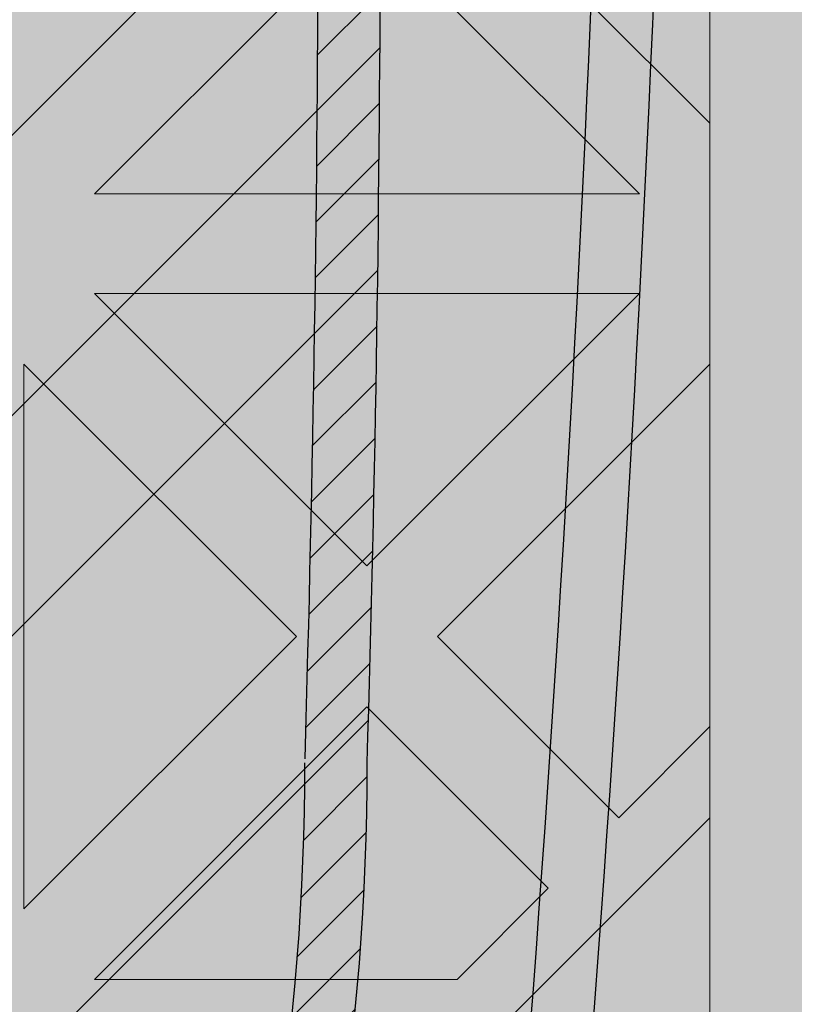
# Model space of a CAD drawing. Units: inches. Extents: x 844 to 2234, y 346 to 1084.
# Tile 11 of 93: x 1125.555 to 1127.536, y 691.183 to 693.702. Entities that reach past the tile are written whole.
import ezdxf

# ---------------------------------------------------------------- set-up
doc = ezdxf.new("R2010")
doc.units = ezdxf.units.IN
doc.header["$MEASUREMENT"] = 0
for name, color, linetype, lineweight in [('A-ANNO-DIMS', 2, 'Continuous', 18), ('furniture', 8, 'Continuous', 18), ('RA-AP-01$0$INT', 35, 'Continuous', 5)]:
    doc.layers.add(name, color=color, linetype=linetype, lineweight=lineweight)
doc.layers.add('RA-AP-01$0$FURN', color=3, linetype='Continuous')
doc.layers.add('RA-AP-01$0$WOOD', color=64, linetype='Continuous')
doc.styles.get("Standard").update_dxf_attribs({"font": 'arial.ttf'})
doc.dimstyles.get("Standard").update_dxf_attribs({"dimtxt": 6, "dimasz": 3, "dimexe": 0.18, "dimexo": 0.0625, "dimgap": 0.09, "dimtad": 0, "dimtih": 1, "dimtoh": 1, "dimdec": 1, "dimzin": 0, "dimdsep": 46, "dimlunit": 3, "dimtxsty": 'Standard', "dimblk": 'ARCHTICK', "dimcen": 0.09, "dimadec": 0, "dimazin": 0, "dimtfac": 1, "dimtdec": 1, "dimtofl": 0, "dimtmove": 0, "dimatfit": 3, "dimfxl": 1, "dimtolj": 1, "dimtzin": 0, "dimarcsym": 0})

# ---------------------------------------------------------------- blocks, each defined once
blk = doc.blocks.new('A$C18D01794')
at = {"layer": 'RA-AP-01$0$INT'}
blk.add_hatch(color=256, dxfattribs=at).paths.add_polyline_path([(4.505206456958071, -6.306712009588038), (5.305206456958072, -6.306712009588038), (5.305206456958072, -7.106712009588038), (5.255206456951893, -7.10671200958804), (5.25520645694868, -6.356712009605972), (4.555206456959269, -6.356712009587461), (4.555206456956052, -7.106712009588038), (4.505206456958073, -7.106712009588038)])
h = blk.add_hatch(color=256, dxfattribs=at)
h.paths.add_polyline_path([(4.585917135068449, -6.356712009588271), (4.555206456959269, -6.35671200958746), (4.555206456959137, -6.387422687716308), (4.874495778835233, -6.706712009592356), (4.90520645695423, -6.676001331474049)])
h.paths.add_polyline_path([(5.255206456948813, -6.387422687716306), (5.255206456948682, -6.356712009605972), (5.224495778822613, -6.356712009605161), (4.905206456953498, -6.676001331474273), (4.935917135072151, -6.706712009592924)])
h.paths.add_polyline_path([(4.935917135072559, -6.706712009592068), (4.905206456953564, -6.737422687710376), (5.255206456951813, -7.087422687708613), (5.255206456951549, -7.026001331471008)])
h.paths.add_polyline_path([(4.555206456956399, -7.026001331471013), (4.555206456956134, -7.087422687708616), (4.905206456953821, -6.737422687710943), (4.874495778835166, -6.70671200959229)])
h = blk.add_hatch(color=256, dxfattribs=at)
h.paths.add_polyline_path([(4.585917135068448, -6.356712009588273), (4.614201406330596, -6.356712009589021), (4.668846067270487, -6.411356670531338), (4.723490728212344, -6.356712009591912), (4.771774999457151, -6.35671200959319), (4.826419660396886, -6.411356670535356), (4.862780050090322, -6.374996280843536), (4.844495778842715, -6.356712009595112), (4.862780050090411, -6.356712009595595), (4.905206456960182, -6.399138416468211), (4.947632863832445, -6.356712009597838), (4.965917135079675, -6.356712009598322), (4.947632863831759, -6.374996280845421), (4.983993253523576, -6.411356670538857), (5.038637914464627, -6.356712009600247), (5.08692218571208, -6.356712009601523), (5.141566846649976, -6.411356670541852), (5.196211507589851, -6.356712009604411), (5.224495778822615, -6.356712009605161), (4.905206456953975, -6.676001331473793)])
h.paths.add_polyline_path([(4.895206456956031, -6.637717060225675), (4.895206456958921, -6.528427738347902), (4.840561796018589, -6.583072399285802)], flags=16)
h.paths.add_polyline_path([(4.915206456955638, -6.637717060226121), (4.969851117895509, -6.583072399288678), (4.915206456957609, -6.528427738348344)], flags=16)
h.paths.add_polyline_path([(4.826419660395175, -6.568930263661755), (4.881064321335613, -6.514285602723745), (4.771774999456703, -6.514285602720857)], flags=16)
h.paths.add_polyline_path([(4.983993253519558, -6.568930263665262), (5.038637914460456, -6.514285602726792), (4.929348592581548, -6.514285602724816)], flags=16)
h.paths.add_polyline_path([(4.881064321336025, -6.494285602723742), (4.826419660397532, -6.439640941782821), (4.771774999457062, -6.494285602720859)], flags=16)
h.paths.add_polyline_path([(4.929348592582019, -6.494285602724817), (5.038637914460982, -6.494285602726792), (4.983993253522945, -6.439640941786327)], flags=16)
h.paths.add_polyline_path([(4.895206456960191, -6.480143467100443), (4.895206456962115, -6.407422687715913), (4.876922185715016, -6.389138416467584), (4.840561796021581, -6.425498806159401)], flags=16)
h.paths.add_polyline_path([(4.915206456958487, -6.480143467100889), (4.969851117899527, -6.425498806162279), (4.933490728206909, -6.389138416468043), (4.9152064569598, -6.40742268771434)], flags=16)
h.paths.add_polyline_path([(4.757632863832376, -6.480143467096812), (4.812277524772842, -6.425498806158772), (4.757632863834348, -6.370854145217844)], flags=16)
h.paths.add_polyline_path([(4.737632863832376, -6.480143467096286), (4.737632863834348, -6.370854145217375), (4.682988202893906, -6.425498806155385)], flags=16)
h.paths.add_polyline_path([(5.05278005008503, -6.480143467103376), (5.052780050087917, -6.370854145224413), (4.998135389146995, -6.425498806162908)], flags=16)
h.paths.add_polyline_path([(5.072780050085024, -6.480143467103744), (5.127424711025931, -6.42549880616527), (5.072780050087916, -6.370854145224832)], flags=16)
h.paths.add_polyline_path([(4.935917135072783, -6.706712009592292), (5.255206456948811, -6.387422687716309), (5.255206456948932, -6.415706958964177), (5.200561796010279, -6.470351619902839), (5.255206456949403, -6.524996280841948), (5.25520645694961, -6.5732805520894), (5.200561796009787, -6.627925213029239), (5.236922185702417, -6.664285602721864), (5.255206456949919, -6.646001331474357), (5.255206456949998, -6.664285602721898), (5.212780050078687, -6.706712009592262), (5.25520645695036, -6.749138416463932), (5.255206456950438, -6.767422687711313), (5.236922185702424, -6.749138416463297), (5.200561796009796, -6.785498806155928), (5.255206456950753, -6.840143467096874), (5.25520645695096, -6.888427738341682), (5.200561796010322, -6.943072399282328), (5.255206456951428, -6.997717060223427), (5.255206456951547, -7.026001331471006)])
h.paths.add_polyline_path([(5.042988202883395, -6.785498806155427), (5.097632863823085, -6.840143467095101), (5.097632863822622, -6.730854145216193)], flags=16)
h.paths.add_polyline_path([(5.028846067259663, -6.771356670531693), (5.083490728198774, -6.716712009592573), (4.974201406321001, -6.716712009593042)], flags=16)
h.paths.add_polyline_path([(5.117632863823087, -6.840143467095186), (5.172277524762331, -6.785498806155926), (5.11763286382262, -6.730854145216225)], flags=16)
h.paths.add_polyline_path([(5.08349072819877, -6.696712009593886), (5.028846067259652, -6.642067348654775), (4.974201406320998, -6.696712009593438)], flags=16)
h.paths.add_polyline_path([(5.131774999446817, -6.854285602718917), (5.186419660386065, -6.799640941779662), (5.241064321325782, -6.854285602719365)], flags=17)
h.paths.add_polyline_path([(5.131774999446228, -6.716712009592374), (5.186419660386065, -6.771356670532194), (5.222780050079488, -6.734996280838764), (5.204495778832781, -6.716712009592063)], flags=16)
h.paths.add_polyline_path([(5.097632863822613, -6.682569873970264), (5.097632863823061, -6.573280552091354), (5.042988202883383, -6.627925213031044)], flags=16)
h.paths.add_polyline_path([(5.131774999446899, -6.874285602718915), (5.241064321325809, -6.874285602719364), (5.186419660386591, -6.928930263658598)], flags=17)
h.paths.add_polyline_path([(5.131774999446226, -6.696712009594078), (5.204495778830767, -6.696712009594374), (5.22278005007868, -6.67842773834687), (5.186419660386049, -6.642067348654249)], flags=16)
h.paths.add_polyline_path([(5.11763286382262, -6.682569873970225), (5.17227752476232, -6.627925213030515), (5.117632863823064, -6.573280552091267)], flags=16)
h.paths.add_polyline_path([(5.186419660386069, -6.613783077405491), (5.241064321325754, -6.559138416465795), (5.131774999446791, -6.559138416466263)], flags=16)
h.paths.add_polyline_path([(5.131774999446872, -6.539138416466263), (5.24106432132578, -6.539138416465794), (5.186419660386554, -6.484493755526573)], flags=16)
h.paths.add_polyline_path([(5.255206456951811, -7.08742268770861), (5.255206456951895, -7.106712009588038), (4.555206456956052, -7.106712009588038), (4.555206456956136, -7.087422687708617), (4.905206456953973, -6.737422687710788)])
h.paths.add_polyline_path([(4.983993253513404, -6.8444937555241), (4.92934859257295, -6.899138416462108), (5.03863791445186, -6.899138416465014)], flags=16)
h.paths.add_polyline_path([(4.969851117889988, -6.83035161990006), (4.915206456952556, -6.775706958960171), (4.915206456949648, -6.884996280837944)], flags=16)
h.paths.add_polyline_path([(4.929348592572535, -6.919138416462105), (4.983993253511019, -6.973783077403037), (5.038637914451496, -6.919138416465012)], flags=16)
h.paths.add_polyline_path([(5.052780050074912, -6.93328055208906), (4.998135389134438, -6.987925213027088), (5.052780050072919, -7.042569873968025)], flags=16)
h.paths.add_polyline_path([(5.07278005007491, -6.933280552089588), (5.072780050072918, -7.042569873968497), (5.127424711013374, -6.987925213030498)], flags=16)
h.paths.add_polyline_path([(4.89520645695295, -6.775706958959721), (4.840561796013067, -6.830351619897157), (4.895206456950961, -6.884996280837494)], flags=16)
h.paths.add_polyline_path([(4.915206456948365, -6.933280552085403), (4.915206456946434, -7.006001331471951), (4.933490728192729, -7.024285602719066), (4.969851117886972, -6.987925213026453)], flags=16)
h.paths.add_polyline_path([(4.881064321327021, -6.899138416461022), (4.82641966038902, -6.84449375552057), (4.771774999448108, -6.899138416459029)], flags=16)
h.paths.add_polyline_path([(4.895206456950073, -6.933280552084951), (4.840561796009022, -6.987925213023558), (4.876922185700835, -7.024285602716997), (4.895206456948749, -7.006001331469487)], flags=16)
h.paths.add_polyline_path([(4.983993253510392, -7.0020673486505), (4.947632863816944, -7.038427738342319), (4.965917135064043, -7.05671200959023), (5.038637914448995, -7.056712009591555)], flags=16)
h.paths.add_polyline_path([(4.881064321326543, -6.91913841646102), (4.771774999447578, -6.919138416459031), (4.826419660385607, -6.973783077399508)], flags=16)
h.paths.add_polyline_path([(4.905206456946447, -7.014285602717636), (4.862780050074785, -7.056712009588352), (4.947632863816685, -7.056712009589775)], flags=16)
h.paths.add_polyline_path([(5.14156684663679, -7.002067348654549), (5.086922185696452, -7.056712009592438), (5.196211507574223, -7.056712009594425)], flags=16)
h.paths.add_polyline_path([(4.8264196603837, -7.002067348646972), (4.771774999442643, -7.056712009585575), (4.8444957788276, -7.056712009587508), (4.862780050075511, -7.038427738340416)], flags=16)
h.paths.add_polyline_path([(4.812277524760289, -6.98792521302292), (4.757632863822258, -6.933280552082447), (4.757632863819352, -7.042569873961408)], flags=16)
h.paths.add_polyline_path([(4.73763286382226, -6.933280552082079), (4.682988202881349, -6.987925213020536), (4.737632863819352, -7.04256987396099)], flags=16)
h.paths.add_polyline_path([(4.723490728195188, -7.056712009584289), (4.668846067257299, -7.002067348643949), (4.614201406317417, -7.056712009581383)], flags=16)
h.paths.add_polyline_path([(4.597632863829262, -6.706712009592262), (4.555206456957951, -6.664285602721896), (4.555206456958029, -6.646001331474357), (4.573490728205535, -6.664285602721864), (4.609851117898167, -6.627925213029238), (4.555206456958338, -6.573280552089402), (4.555206456958546, -6.524996280841952), (4.60985111789767, -6.470351619902839), (4.555206456959015, -6.415706958964177), (4.555206456959138, -6.387422687716309), (4.874495778835167, -6.70671200959229), (4.5552064569564, -7.026001331471015), (4.555206456956523, -6.997717060223433), (4.609851117897629, -6.94307239928233), (4.555206456956988, -6.888427738341681), (4.555206456957198, -6.840143467096881), (4.609851117898153, -6.78549880615593), (4.573490728205528, -6.749138416463297), (4.555206456957507, -6.76742268771132), (4.555206456957585, -6.749138416463933)])
h.paths.add_polyline_path([(4.712780050085332, -6.730854145216195), (4.712780050084863, -6.840143467095105), (4.767424711024555, -6.785498806155427)], flags=16)
h.paths.add_polyline_path([(4.726922185709173, -6.716712009592573), (4.781566846648288, -6.771356670531693), (4.836211507586949, -6.716712009593043)], flags=16)
h.paths.add_polyline_path([(4.692780050085327, -6.730854145216225), (4.638135389145619, -6.785498806155928), (4.692780050084865, -6.840143467095185)], flags=16)
h.paths.add_polyline_path([(4.726922185709182, -6.696712009593886), (4.836211507586949, -6.696712009593436), (4.7815668466483, -6.642067348654773)], flags=16)
h.paths.add_polyline_path([(4.678637914461726, -6.71671200959237), (4.605917135075169, -6.716712009592063), (4.587632863828464, -6.734996280838766), (4.623993253521887, -6.771356670532195)], flags=16)
h.paths.add_polyline_path([(4.712780050085336, -6.68256987397026), (4.767424711024568, -6.627925213031042), (4.71278005008489, -6.573280552091352)], flags=16)
h.paths.add_polyline_path([(4.678637914461726, -6.696712009594076), (4.623993253521899, -6.642067348654247), (4.587632863829271, -6.67842773834687), (4.605917135077185, -6.696712009594376)], flags=16)
h.paths.add_polyline_path([(4.692780050085336, -6.682569873970228), (4.692780050084889, -6.573280552091267), (4.638135389145632, -6.627925213030515)], flags=16)
h.paths.add_polyline_path([(4.623993253521885, -6.799640941779662), (4.678637914461131, -6.854285602718915), (4.56934859258217, -6.854285602719365)], flags=17)
h.paths.add_polyline_path([(4.623993253521901, -6.613783077405509), (4.678637914461158, -6.559138416466263), (4.569348592582195, -6.559138416465795)], flags=16)
h.paths.add_polyline_path([(4.678637914461051, -6.874285602718915), (4.623993253521361, -6.928930263658598), (4.569348592582143, -6.874285602719364)], flags=17)
h.paths.add_polyline_path([(4.678637914461076, -6.539138416466263), (4.623993253521399, -6.484493755526573), (4.569348592582167, -6.539138416465796)], flags=16)
h = blk.add_hatch(color=256, dxfattribs=at)
h.paths.add_polyline_path([(5.028846067259997, -6.642067348655121), (4.974201406321342, -6.696712009593783), (5.083490728199115, -6.69671200959423)])
h.paths.add_polyline_path([(4.974201406321344, -6.716712009593388), (5.028846067260004, -6.771356670532039), (5.083490728199117, -6.716712009592919)])
h.paths.add_polyline_path([(5.042988202883738, -6.785498806155768), (5.097632863823428, -6.840143467095449), (5.097632863822963, -6.73085414521654)])
h.paths.add_polyline_path([(5.117632863822961, -6.730854145216568), (5.117632863823428, -6.840143467095531), (5.172277524762674, -6.785498806156272)])
h.paths.add_polyline_path([(5.131774999446572, -6.716712009592718), (5.186419660386406, -6.77135667053254), (5.222780050079831, -6.734996280839116), (5.204495778833122, -6.716712009592409)])
h.paths.add_polyline_path([(5.236922185702764, -6.749138416463644), (5.200561796010139, -6.785498806156274), (5.255206456949971, -6.840143467096101), (5.255206456950271, -6.76742268771115)])
h.paths.add_polyline_path([(5.186419660386412, -6.799640941780006), (5.131774999447164, -6.854285602719262), (5.241064321326123, -6.854285602719711)])
h.paths.add_polyline_path([(5.131774999447238, -6.874285602719261), (5.186419660386934, -6.928930263658944), (5.241064321326153, -6.874285602719709)])
h.paths.add_polyline_path([(5.200561796010663, -6.943072399282675), (5.255206456949324, -6.997717060221329), (5.255206456949777, -6.888427738343558)])
h.paths.add_polyline_path([(5.21278005007903, -6.706712009592607), (5.255206456950223, -6.749138416463798), (5.255206456950696, -6.664285602721891)])
h.paths.add_polyline_path([(5.13177499944657, -6.696712009594424), (5.204495778831106, -6.696712009594723), (5.222780050079024, -6.678427738347219), (5.186419660386397, -6.642067348654592)])
h.paths.add_polyline_path([(5.117632863823405, -6.573280552091611), (5.117632863822955, -6.682569873970578), (5.172277524762665, -6.627925213030859)])
h.paths.add_polyline_path([(5.042988202883727, -6.627925213031387), (5.097632863822957, -6.682569873970603), (5.097632863823407, -6.573280552091697)])
h.paths.add_polyline_path([(5.131774999447135, -6.559138416466609), (5.186419660386394, -6.613783077405857), (5.241064321326097, -6.559138416466144)])
h.paths.add_polyline_path([(5.200561796010128, -6.627925213029584), (5.236922185702758, -6.664285602722211), (5.255206456950264, -6.646001331474705), (5.255206456949948, -6.573280552089752)])
h.paths.add_polyline_path([(5.186419660386895, -6.484493755526919), (5.131774999447213, -6.539138416466609), (5.241064321326127, -6.539138416466142)])
h.paths.add_polyline_path([(5.200561796010624, -6.470351619903183), (5.255206456949745, -6.524996280842298), (5.255206456949276, -6.415706958964523)])
for p, q in [((5.255206456951895, -7.106712009588038), (5.255206456948681, -6.356712009605972)), ((5.25520645694988, -6.74913841646345), (5.255206456950353, -6.664285602721543)), ((4.935917135072783, -6.706712009592292), (5.255206456951548, -7.026001331471007)), ((5.212780050078687, -6.706712009592262), (5.25520645694988, -6.74913841646345)), ((5.131774999446229, -6.716712009592372), (5.186419660386063, -6.771356670532195)), ((5.204495778831181, -6.716712009592063), (5.131774999446229, -6.716712009592372)), ((5.204495778832774, -6.716712009592056), (5.222780050080282, -6.73499628083956)), ((5.11763286382262, -6.730854145216223), (5.172277524762331, -6.785498806155928)), ((5.117632863823085, -6.840143467095186), (5.11763286382262, -6.730854145216223)), ((5.186419660386062, -6.771356670532195), (5.222780050078687, -6.734996280839565)), ((5.200561796009796, -6.78549880615593), (5.236922185702423, -6.749138416463297)), ((5.255206456949928, -6.767422687710803), (5.236922185702423, -6.749138416463296)), ((5.236922185702423, -6.749138416463297), (5.25520645694988, -6.767422687710757)), ((5.255206456949927, -6.767422687710803), (5.255206456949628, -6.840143467095755)), ((5.117632863823085, -6.840143467095186), (5.172277524762331, -6.785498806155928)), ((5.255206456949628, -6.840143467095755), (5.200561796009796, -6.785498806155928)), ((5.131774999446817, -6.854285602718915), (5.186419660386065, -6.799640941779662)), ((5.24106432132578, -6.854285602719365), (5.186419660386065, -6.799640941779662)), ((5.131774999446817, -6.854285602718915), (5.24106432132578, -6.854285602719365)), ((5.131774999446899, -6.874285602718915), (5.241064321325809, -6.874285602719364)), ((5.186419660386587, -6.928930263658596), (5.131774999446899, -6.874285602718915)), ((5.241064321325809, -6.874285602719364), (5.186419660386589, -6.928930263658598)), ((5.255206456949429, -6.888427738343214), (5.200561796010322, -6.943072399282328)), ((5.255206456949433, -6.888427738343212), (5.255206456948982, -6.997717060220983))]:
    blk.add_line(p, q, dxfattribs=at)
blk = doc.blocks.new('A$C32926AE1')
at = {"layer": 'RA-AP-01$0$WOOD'}
h = blk.add_hatch(color=256, dxfattribs=at)
h.dxf.hatch_style = 1
h.paths.add_polyline_path([(5.157430609644524, 4.573483066760929, -0.1009492694046607), (5.155401577623758, 4.593365984175333, -0.1842662638101597), (5.172249623284174, 4.638795604568598, 0.2056608120311276), (5.179560981299304, 4.661316324430096, 0.3614336704623542), (5.134352340494423, 4.706524965234944, 0.2056608120311297), (5.111831620632933, 4.699213607219793, -0.1842662638101113), (5.066402000239693, 4.682365561559342, -0.1055311479399994), (5.045656153913092, 4.68467289944697, 0.1567636581983829), (4.763886414745334, 4.684672899446966, -0.1055311479399895), (4.743140568418733, 4.68236556155934, -0.1842662638100833), (4.6977109480255, 4.69921360721979, 0.2056608120302612), (4.675190228164109, 4.706524965234949, 0.3614336704708441), (4.629981587358889, 4.66131632442871, 0.2056608120245944), (4.637292945374126, 4.638795604567974, -0.1842662638101024), (4.654140991034615, 4.59336598417475, -0.1009492694055169), (4.652111959013835, 4.573483066760181, 0.021410119221476), (4.629748025606143, 4.156712009541676, 0.0214101192214795), (4.652111959013809, 3.739940952323101, -0.1009492694059586), (4.654140991034615, 3.720058034908448, -0.1842662638100975), (4.637292945374126, 3.674628414515226, 0.2056608120245705), (4.629981587358889, 3.652107694654492, 0.3614336704708879), (4.675190228164113, 3.606899053848249, 0.2056608120302384), (4.697710948025501, 3.614210411863408, -0.1842662638100995), (4.743140568418738, 3.63105845752386, -0.1055311479402541), (4.763886414745388, 3.628751119636215, 0.1567636581983776), (5.045656153913137, 3.628751119636244, -0.1055311479397538), (5.066402000239692, 3.631058457523857, -0.1842662638101067), (5.111831620632931, 3.614210411863407, 0.2056608120310924), (5.134352340494417, 3.606899053848256, 0.3614336704624001), (5.179560981299307, 3.652107694653103, 0.2056608120311314), (5.172249623284175, 3.6746284145146, -0.1842662638101402), (5.155401577623758, 3.72005803490786, -0.1009492694051366), (5.15743060964455, 3.739940952322354, 0.0214101192215073), (5.179794543052287, 4.156712009541468, 0.0214101192215252)])
h.paths.add_polyline_path([(4.639748609479751, 4.156712009541513, 0.0213537860821624), (4.661970494867118, 3.741887061152232, -0.094075836301374), (4.664143710413708, 3.7196126951003, -0.1824818158568985), (4.644813765429836, 3.668037719127816, 0.2056608120245319), (4.639939526753007, 3.653023905887301, 0.3614336704710246), (4.676106439397173, 3.616856993242342, 0.2056608120302234), (4.691120252638095, 3.621731231919122, -0.1824818158602558), (4.742695228611606, 3.641061176902986, -0.1029891339458722), (4.766991894714349, 3.638256818950944, 0.156709409989566), (5.042550673941472, 3.638256818950105, -0.102989133958497), (5.066847340047078, 3.641061176902949, -0.1824818158594995), (5.118422316020358, 3.621731231919103, 0.2056608120311416), (5.133436129261316, 3.616856993242346, 0.3614336704621468), (5.169603041905217, 3.653023905886178, 0.2056608120310986), (5.164728803228477, 3.668037719127177, -0.1824818158565612), (5.145398858244737, 3.719612695099578, -0.0940758363009313), (5.147572073791232, 3.741887061151398, 0.0213537860822023), (5.169793959178681, 4.156712009541451, 0.0213537860822226), (5.147572073791203, 4.571536957931898, -0.0940758363005034), (5.145398858244737, 4.59381132398362, -0.1824818158565587), (5.164728803228476, 4.645386299956021, 0.2056608120311045), (5.169603041905216, 4.66040011319702, 0.3614336704621845), (5.133436129261313, 4.696567025840856, 0.2056608120310773), (5.118422316020359, 4.691692787164098, -0.182481815859508), (5.066847340047078, 4.67236284218025, -0.1029891339584606), (5.04255067394148, 4.675167200133092, 0.156709409989566), (4.766991894714357, 4.675167200132257, -0.1029891339458842), (4.742695228611611, 4.672362842180213, -0.1824818158602725), (4.691120252638095, 4.691692787164077, 0.2056608120302152), (4.676106439397174, 4.696567025840858, 0.3614336704710363), (4.639939526753005, 4.660400113195899, 0.2056608120245495), (4.644813765429837, 4.645386299955384, -0.1824818158568934), (4.664143710413708, 4.593811323982902, -0.0940758363009187), (4.661970494867149, 4.571536957931074, 0.021353786082177)], flags=16)
h.paths.add_polyline_path([(5.129794543052235, 4.432167055276933, -0.0141661062790638), (5.130152669293814, 4.156927903047693, -0.0141661062790647), (5.129794543052234, 3.881688750818433, -0.0785247771143638), (5.10979738006795, 3.755143611847103, 0.0945969212073497), (5.105408519571111, 3.717898134952927, 0.1043170707844957), (5.116074640131521, 3.670385395016088, 0.1043170707864965), (5.068561900193738, 3.681051515576561, 0.09459692119553), (5.031316423304057, 3.676662655080835, -0.1580239521427272), (4.778226145355827, 3.676662655080367, 0.0945969211986668), (4.740980668464973, 3.681051515576592, 0.1043170707882822), (4.693467928526415, 3.670385395015844, 0.1043170707867916), (4.704134049087309, 3.717898134953662, 0.0945969211972894), (4.69974518859162, 3.755143611844042, -0.0785247771163196), (4.679748025606343, 3.881688750818406, -0.0141661062790663), (4.679389899364763, 4.156927903047693, -0.0141661062790672), (4.679748025606343, 4.432167055276998, -0.0785247771163064), (4.699745188591625, 4.55871219425134, 0.094596921197333), (4.704134049087308, 4.595957671141738, 0.1043170707867205), (4.693467928526416, 4.643470411079523, 0.1043170707882628), (4.740980668464965, 4.632804290518776, 0.0945969211988114), (4.778226145355874, 4.637193151015016, -0.158023952142669), (5.031316423304015, 4.637193151014546, 0.0945969211956361), (5.068561900193736, 4.632804290518806, 0.1043170707864979), (5.11607464013152, 4.643470411079278, 0.1043170707844617), (5.105408519571112, 4.595957671142455, 0.0945969212074597), (5.109797380067959, 4.558712194248236, -0.0785247771143467)], flags=0)
h.paths.add_polyline_path([(5.119794532311105, 4.432259799204851, -0.0142000800617244), (5.120156169157484, 4.156927903047701, -0.0142000800617277), (5.119794532311105, 3.881596006890482, -0.0784894509520253), (5.100273383573699, 3.758192358677797, 0.0940138827242913), (5.095413455884425, 3.717477693979438, 0.0606271852308753), (5.099615656341024, 3.686844378806616, 0.0606271852322524), (5.068982341167493, 3.691046579263239, 0.0940138827010453), (5.028267676478798, 3.686186651576848, -0.1580706864508061), (4.781274892180912, 3.686186651576435, 0.0940138827026903), (4.740560227491556, 3.691046579263279, 0.0606271852339895), (4.709926912317155, 3.686844378806508, 0.0606271852329405), (4.714129112773991, 3.717477693980356, 0.094013882701304), (4.709269185087677, 3.758192358669163, -0.0784894509577193), (4.689748036347473, 3.881596006890469, -0.014200080061729), (4.689386399501094, 4.156927903047709, -0.0142000800617217), (4.689748036347473, 4.432259799204808, -0.078489450957724), (4.709269185087651, 4.555663447426125, 0.0940138827014585), (4.714129112773992, 4.596378112114996, 0.0606271852329731), (4.709926912317154, 4.62701142728886, 0.0606271852340196), (4.74056022749157, 4.622809226832087, 0.0940138827024997), (4.781274892180847, 4.627669154518912, -0.1580706864508359), (5.028267676478777, 4.627669154518526, 0.0940138827010946), (5.068982341167492, 4.622809226832129, 0.060627185232254), (5.099615656341024, 4.627011427288751, 0.0606271852308727), (5.095413455884425, 4.59637811211593, 0.0940138827241088), (5.100273383573675, 4.555663447417647, -0.0784894509520978)], flags=0)
h.paths.add_polyline_path([(5.06978912287499, 4.430218106756144, -0.014241683694547), (5.070173729147532, 4.156927903047672, -0.0142416836945458), (5.06978912287499, 3.883637699339223, -0.0800609523125196), (5.052662118612511, 3.773463122773442, 0.0526421978001116), (5.04590916754064, 3.740550867606997, 0.0526421977992423), (5.012996912374707, 3.73379791653534, -0.1583028414718258), (4.796545656286308, 3.73379791653451, 0.0526421978034211), (4.763633401117837, 3.740550867607021, 0.0526421978018622), (4.756880450045755, 3.773463122774558, -0.0800609523117106), (4.739753445783639, 3.883637699339268, -0.0142416836945435), (4.739368839511098, 4.156927903047671, -0.0142416836945477), (4.739753445783639, 4.430218106756155, -0.0800609523116345), (4.75688045004574, 4.540392683320762, 0.052642197801941), (4.763633401117837, 4.573304938488346, 0.0526421978035071), (4.796545656286361, 4.580057889560873, -0.1583028414717561), (5.012996912374669, 4.580057889560039, 0.0526421977993048), (5.04590916754064, 4.57330493848837, 0.0526421978002057), (5.052662118612529, 4.540392683321868, -0.080060952312477)], flags=0)
h.paths.add_polyline_path([(5.049789715110557, 4.43038092723357, -0.0143097550741839), (5.05018085590259, 4.156927903047715, -0.0143097550741854), (5.049789715110558, 3.883474878861827, -0.0800685599149176), (5.03362098255317, 3.779581877367999, 0.0306258898956367), (5.028241146483733, 3.758218888663947, 0.0306258898977031), (5.006878157778253, 3.75283905259408, -0.1583983521624096), (4.802664410878162, 3.752839052594731, 0.0306258898946014), (4.781301422174808, 3.758218888663924, 0.0306258898967912), (4.775921586105202, 3.779581877368794, -0.080068559914251), (4.759752853548071, 3.883474878861786, -0.0143097550741854), (4.759361712756037, 4.156927903047671, -0.0143097550741854), (4.759752853548071, 4.430380927233557, -0.0800685599142479), (4.775921586105193, 4.534273928726546, 0.0306258898968306), (4.781301422174808, 4.555636917431444, 0.0306258898945754), (4.802664410878143, 4.561016753500631, -0.1583983521624168), (5.006878157778244, 4.561016753501291, 0.0306258898977177), (5.028241146483733, 4.555636917431421, 0.0306258898958182), (5.03362098255321, 4.534273928727244, -0.080068559914796)], flags=0)
h.paths.add_polyline_path([(4.999766070382627, 4.428171244713864, -0.0143443147609634), (5.000198441819402, 4.156927903047689, -0.0143443147609612), (4.999766070382627, 3.885684561381556, -0.0784641635803329), (4.987356730658798, 3.799103304488872, -0.1506053783831347), (4.822185837999821, 3.79910330448882, -0.0784641635803318), (4.809776498276007, 3.885684561381509, -0.014344314760963), (4.809344126839227, 4.156927903047677, -0.0143443147609645), (4.809776498276007, 4.428171244713873, -0.0784641635803192), (4.822185837999822, 4.514752501606549, -0.1506053783831338), (4.987356730658798, 4.514752501606494, -0.078464163580285)], flags=0)
h.paths.add_polyline_path([(4.979755254238824, 4.42764379880488, -0.0143772539198268), (4.980205517789977, 4.156927903047693, -0.0143772539198275), (4.979755254238824, 3.886212007290489, -0.0689242507424422), (4.971183264704897, 3.815276770442801, -0.1296645318904179), (4.838359303953726, 3.815276770442746, -0.0689242507424186), (4.829787314419809, 3.886212007290419, -0.0143772539198292), (4.829337050868653, 4.156927903047653, -0.0143772539198325), (4.829787314419809, 4.427643798804946, -0.0689242507424211), (4.838359303953725, 4.498579035652621, -0.1296645318904187), (4.971183264704897, 4.498579035652565, -0.0689242507424401)], flags=0)
h = blk.add_hatch(color=256, dxfattribs=at)
h.dxf.hatch_style = 1
h.paths.add_polyline_path([(5.145398858244737, 4.59381132398362, -0.1824818158565616), (5.164728803228476, 4.645386299956021, 0.2056608120311045), (5.169603041905216, 4.66040011319702, 0.3614336704621845), (5.133436129261313, 4.696567025840856, 0.2056608120310773), (5.118422316020359, 4.691692787164098, -0.182481815859508), (5.066847340047078, 4.67236284218025, -0.1029891339584606), (5.04255067394148, 4.675167200133092, 0.156709409989566), (4.766991894714357, 4.675167200132257, -0.1029891339458842), (4.742695228611611, 4.672362842180213, -0.1824818158602725), (4.691120252638095, 4.691692787164077, 0.2056608120302152), (4.676106439397174, 4.696567025840858, 0.3614336704710363), (4.639939526753005, 4.660400113195899, 0.2056608120245495), (4.644813765429837, 4.645386299955384, -0.1824818158568934), (4.664143710413708, 4.593811323982902, -0.0940758363009187), (4.661970494867149, 4.571536957931074, 0.0213537860821772), (4.639748609479751, 4.156712009541507, 0.0213537860821625), (4.661970494867119, 3.741887061152226, -0.0940758363013071), (4.664143710413708, 3.719612695100309, -0.1824818158569294), (4.644813765429836, 3.668037719127816, 0.2056608120245319), (4.639939526753007, 3.653023905887301, 0.3614336704710246), (4.676106439397173, 3.616856993242342, 0.2056608120302234), (4.691120252638095, 3.621731231919122, -0.1824818158602558), (4.742695228611606, 3.641061176902986, -0.1029891339458722), (4.766991894714349, 3.638256818950944, 0.156709409989566), (5.042550673941472, 3.638256818950105, -0.102989133958497), (5.066847340047078, 3.641061176902949, -0.1824818158594995), (5.118422316020358, 3.621731231919103, 0.2056608120311416), (5.133436129261316, 3.616856993242346, 0.3614336704621468), (5.169603041905217, 3.653023905886178, 0.2056608120310986), (5.164728803228477, 3.668037719127177, -0.1824818158565612), (5.145398858244737, 3.719612695099578, -0.0940758363009313), (5.147572073791232, 3.741887061151398, 0.0213537860822023), (5.169793959178681, 4.156712009541451, 0.0213537860822226), (5.147572073791203, 4.571536957931898, -0.0940758363004996)])
h.paths.add_polyline_path([(5.109797380067958, 4.55871219424824, -0.0785247771143472), (5.129794543052234, 4.432167055276936, -0.0141661062790644), (5.130152669293814, 4.156927903047685, -0.014166106279066), (5.129794543052234, 3.881688750818401, -0.0785247771143517), (5.109797380067946, 3.755143611847092, 0.0945969212073132), (5.105408519571111, 3.717898134952929, 0.1043170707844995), (5.116074640131521, 3.670385395016088, 0.1043170707864965), (5.068561900193738, 3.681051515576561, 0.09459692119553), (5.031316423304057, 3.676662655080835, -0.1580239521427272), (4.778226145355827, 3.676662655080367, 0.0945969211986668), (4.740980668464973, 3.681051515576592, 0.1043170707882822), (4.693467928526415, 3.670385395015844, 0.1043170707867916), (4.704134049087309, 3.717898134953662, 0.0945969211972894), (4.69974518859162, 3.755143611844042, -0.0785247771163196), (4.679748025606343, 3.881688750818406, -0.0141661062790663), (4.679389899364763, 4.156927903047693, -0.0141661062790672), (4.679748025606343, 4.432167055276998, -0.0785247771163064), (4.699745188591625, 4.55871219425134, 0.094596921197333), (4.704134049087308, 4.595957671141738, 0.1043170707867205), (4.693467928526416, 4.643470411079523, 0.1043170707882628), (4.740980668464965, 4.632804290518776, 0.0945969211988114), (4.778226145355874, 4.637193151015016, -0.158023952142669), (5.031316423304015, 4.637193151014546, 0.0945969211956361), (5.068561900193736, 4.632804290518806, 0.1043170707864979), (5.11607464013152, 4.643470411079278, 0.1043170707844617), (5.105408519571112, 4.595957671142455, 0.0945969212074504)], flags=16)
h.paths.add_polyline_path([(5.100273383573655, 4.55566344741771, -0.0784894509521388), (5.119794532311105, 4.432259799204852, -0.0142000800617252), (5.120156169157484, 4.156927903047686, -0.014200080061726), (5.119794532311105, 3.881596006890502, -0.0784894509520446), (5.100273383573696, 3.758192358677786, 0.0940138827242721), (5.095413455884425, 3.717477693979436, 0.0606271852308692), (5.099615656341024, 3.686844378806616, 0.0606271852322522), (5.068982341167493, 3.691046579263239, 0.0940138827010453), (5.028267676478798, 3.686186651576848, -0.1580706864508061), (4.781274892180912, 3.686186651576435, 0.0940138827026903), (4.740560227491556, 3.691046579263279, 0.0606271852339895), (4.709926912317155, 3.686844378806508, 0.0606271852329405), (4.714129112773991, 3.717477693980356, 0.094013882701304), (4.709269185087677, 3.758192358669163, -0.0784894509577193), (4.689748036347473, 3.881596006890469, -0.014200080061729), (4.689386399501094, 4.156927903047709, -0.0142000800617217), (4.689748036347473, 4.432259799204808, -0.078489450957724), (4.709269185087651, 4.555663447426125, 0.0940138827014585), (4.714129112773992, 4.596378112114996, 0.0606271852329731), (4.709926912317154, 4.62701142728886, 0.0606271852340196), (4.74056022749157, 4.622809226832087, 0.0940138827024997), (4.781274892180847, 4.627669154518912, -0.1580706864508359), (5.028267676478777, 4.627669154518526, 0.0940138827010946), (5.068982341167492, 4.622809226832129, 0.060627185232254), (5.099615656341024, 4.627011427288751, 0.0606271852308727), (5.095413455884425, 4.59637811211593, 0.094013882723957)], flags=0)
h.paths.add_polyline_path([(5.04590916754064, 4.57330493848837, 0.0526421978002057), (5.052662118612529, 4.540392683321868, -0.0800609523124783), (5.06978912287499, 4.430218106756142, -0.0142416836945469), (5.070173729147532, 4.156927903047672, -0.0142416836945458), (5.06978912287499, 3.883637699339223, -0.0800609523125196), (5.052662118612511, 3.773463122773442, 0.0526421978001116), (5.04590916754064, 3.740550867606997, 0.0526421977992423), (5.012996912374707, 3.73379791653534, -0.1583028414718258), (4.796545656286308, 3.73379791653451, 0.0526421978034211), (4.763633401117837, 3.740550867607021, 0.0526421978018622), (4.756880450045755, 3.773463122774558, -0.0800609523117106), (4.739753445783639, 3.883637699339268, -0.0142416836945435), (4.739368839511098, 4.156927903047671, -0.0142416836945477), (4.739753445783639, 4.430218106756155, -0.0800609523116345), (4.75688045004574, 4.540392683320762, 0.052642197801941), (4.763633401117837, 4.573304938488346, 0.0526421978035071), (4.796545656286361, 4.580057889560873, -0.1583028414717561), (5.012996912374669, 4.580057889560039, 0.0526421977993048)], flags=0)
h.paths.add_polyline_path([(5.028241146483733, 4.555636917431422, 0.0306258898956949), (5.033620982553182, 4.534273928727329, -0.0800685599148649), (5.049789715110557, 4.430380927233569, -0.0143097550741839), (5.05018085590259, 4.156927903047715, -0.0143097550741854), (5.049789715110558, 3.883474878861827, -0.0800685599149176), (5.03362098255317, 3.779581877367999, 0.0306258898956367), (5.028241146483733, 3.758218888663947, 0.0306258898977031), (5.006878157778253, 3.75283905259408, -0.1583983521624096), (4.802664410878162, 3.752839052594731, 0.0306258898946014), (4.781301422174808, 3.758218888663924, 0.0306258898967912), (4.775921586105202, 3.779581877368794, -0.080068559914251), (4.759752853548071, 3.883474878861786, -0.0143097550741854), (4.759361712756037, 4.156927903047671, -0.0143097550741854), (4.759752853548071, 4.430380927233557, -0.0800685599142479), (4.775921586105193, 4.534273928726546, 0.0306258898968306), (4.781301422174808, 4.555636917431444, 0.0306258898945754), (4.802664410878143, 4.561016753500631, -0.1583983521624168), (5.006878157778244, 4.561016753501291, 0.0306258898977174)], flags=0)
h.paths.add_polyline_path([(4.987356730658798, 4.514752501606494, -0.0784641635803018), (4.999766070382627, 4.428171244713845, -0.0143443147609637), (5.000198441819402, 4.156927903047665, -0.0143443147609622), (4.999766070382628, 3.885684561381514, -0.0784641635802952), (4.987356730658797, 3.799103304488872, -0.1506053783831338), (4.822185837999821, 3.799103304488819, -0.0784641635803342), (4.809776498276007, 3.885684561381512, -0.0143443147609628), (4.809344126839227, 4.156927903047676, -0.0143443147609646), (4.809776498276007, 4.428171244713873, -0.0784641635803192), (4.822185837999822, 4.514752501606549, -0.1506053783831338)], flags=0)
h.paths.add_polyline_path([(4.971183264704897, 4.498579035652566, -0.0689242507424384), (4.979755254238824, 4.427643798804883, -0.0143772539198276), (4.980205517789977, 4.15692790304768, -0.0143772539198258), (4.979755254238823, 3.88621200729051, -0.0689242507424628), (4.971183264704897, 3.815276770442801, -0.129664531890417), (4.838359303953726, 3.815276770442746, -0.0689242507424186), (4.829787314419809, 3.886212007290419, -0.0143772539198292), (4.829337050868653, 4.156927903047653, -0.0143772539198325), (4.829787314419809, 4.427643798804946, -0.0689242507424211), (4.838359303953725, 4.498579035652621, -0.1296645318904187)], flags=0)
h = blk.add_hatch(dxfattribs=at)
h.set_pattern_fill('ANSI31', color=256, scale=0.05, style=0)
h.set_pattern_definition([(45, (0, 0), (-0.0044194173824159, 0.0044194173824159), [])])
h.paths.add_polyline_path([(5.130152669293814, 4.156927903047704, 0.0141661062790657), (5.129794543052234, 4.432167055276982, 0.0777827904001433), (5.110168979996553, 4.557559993161921, -0.0976515123401879), (5.105408519571111, 4.595957671142454, -0.1043170707844687), (5.116074640131522, 4.64347041107928), (5.099615656341024, 4.627011427288751, 0.0606271852308727), (5.095413455884425, 4.59637811211593, 0.0940138827241088), (5.100273383573675, 4.555663447417647, -0.0784894509520972), (5.119794532311105, 4.432259799204852, -0.0142000800617252), (5.120156169157484, 4.156927903047686, -0.014200080061726), (5.119794532311105, 3.881596006890502, -0.0784894509520446), (5.100273383573696, 3.758192358677786, 0.0940138827242721), (5.095413455884425, 3.717477693979436, 0.0606271852308692), (5.099615656341024, 3.686844378806616), (5.116074640131519, 3.67038539501609, -0.1043170707844594), (5.105408519571112, 3.717898134952912, -0.0976515123401594), (5.11016897999655, 3.756295812933435, 0.0777827904001654), (5.129794543052234, 3.881688750818409, 0.0141661062790665)])
h.paths.add_polyline_path([(5.030164222210597, 3.676291055149937, -0.0976515123472002), (5.068561900193739, 3.681051515576561, -0.1043170707864927), (5.116074640131521, 3.670385395016088), (5.099615656341024, 3.686844378806616, 0.0606271852322522), (5.068982341167493, 3.691046579263239, 0.0940138827010453), (5.028267676478798, 3.686186651576848, -0.1580706864508061), (4.781274892180912, 3.686186651576435, 0.0940138827026903), (4.740560227491556, 3.691046579263279, 0.0606271852339913), (4.709926912317154, 3.686844378806508), (4.693467928526416, 3.670385395015845, -0.1043170707882796), (4.740980668464973, 3.681051515576592, -0.0976515123427246), (4.779378346446416, 3.676291055150394, 0.156512506893803)])
h.paths.add_polyline_path([(4.689748036347473, 3.881596006890472, -0.014200080061729), (4.689386399501094, 4.156927903047712, -0.0142000800617195), (4.689748036347473, 4.432259799204768, -0.078489450957742), (4.709269185087648, 4.555663447426114, 0.0940138827014821), (4.714129112773992, 4.596378112114995, 0.0606271852329748), (4.709926912317154, 4.62701142728886), (4.693467928526414, 4.643470411079524, -0.1043170707867939), (4.704134049087309, 4.595957671141706, -0.09765151234893), (4.699373588660725, 4.557559993157876, 0.0777827903975372), (4.679748025606343, 4.432167055276987, 0.0141661062790675), (4.679389899364763, 4.156927903047675, 0.0141661062790641), (4.679748025606343, 3.88168875081843, 0.0777827903975637), (4.699373588660724, 3.756295812937497, -0.0976515123490278), (4.704134049087308, 3.717898134953629, -0.1043170707867196), (4.693467928526416, 3.670385395015845), (4.709926912317155, 3.686844378806508, 0.0606271852329413), (4.714129112773991, 3.717477693980357, 0.0940138827013084), (4.709269185087676, 3.758192358669166, -0.0784894509577192)])
h.paths.add_polyline_path([(4.779378346446434, 4.63756475094498, -0.0976515123427943), (4.740980668464964, 4.632804290518776, -0.1043170707882609), (4.693467928526416, 4.643470411079523), (4.709926912317154, 4.62701142728886, 0.0606271852340196), (4.74056022749157, 4.622809226832087, 0.0940138827024997), (4.781274892180847, 4.627669154518912, -0.1580706864508359), (5.028267676478777, 4.627669154518526, 0.0940138827010946), (5.068982341167492, 4.622809226832129, 0.060627185232254), (5.099615656341024, 4.627011427288751), (5.116074640131521, 4.643470411079279, -0.1043170707865022), (5.068561900193735, 4.632804290518806, -0.0976515123475899), (5.030164222210446, 4.637564750945479, 0.1565125068936924)])
h = blk.add_hatch(dxfattribs=at)
h.set_pattern_fill('ANSI32', color=256, scale=0.2, style=0)
h.set_pattern_definition([(45, (0, 0), (-0.0530330085889911, 0.0530330085889911), []), (45, (0.035355339, 0), (-0.0530330085889911, 0.0530330085889911), [])])
h.paths.add_polyline_path([(5.119794532311105, 4.432259799204823, 0.0777015974868765), (5.10065834347252, 4.554469821747928, -0.0968902511992216), (5.095413455884425, 4.596378112115931, -0.060627185230871), (5.099615656341024, 4.627011427288751, -0.060627185232254), (5.068982341167492, 4.622809226832129, -0.0968902512198245), (5.027074050790956, 4.628054114423209, 0.1564657949319105), (4.782468517866163, 4.628054114422785, -0.0968902512152247), (4.740560227491555, 4.622809226832088, -0.0606271852339878), (4.709926912317155, 4.627011427288859, -0.0606271852329413), (4.714129112773991, 4.596378112115011, -0.0968902512205338), (4.708884225182929, 4.554469821738175, 0.0777015974804443), (4.689748036347473, 4.43225979920482, 0.0142000800617215), (4.689386399501094, 4.156927903047726, 0.0142000800617273), (4.689748036347473, 3.88159600689052, 0.077701597480541), (4.708884225182985, 3.759385984357019, -0.096890251220082), (4.714129112773992, 3.717477693980371, -0.0606271852329731), (4.709926912317154, 3.686844378806507, -0.060627185233988), (4.740560227491554, 3.691046579263279, -0.0968902512152569), (4.782468517866175, 3.685801691672578, 0.1564657949319236), (5.027074050790988, 3.685801691672169, -0.0968902512197451), (5.068982341167491, 3.691046579263239, -0.0606271852322557), (5.099615656341024, 3.686844378806616, -0.0606271852308727), (5.095413455884425, 3.717477693979438, -0.0968902511991229), (5.100658343472507, 3.7593859843474, 0.0777015974868745), (5.119794532311105, 3.8815960068905, 0.014200080061726), (5.120156169157484, 4.156927903047685, 0.0142000800617238)])
h.paths.add_polyline_path([(5.070173729147531, 4.156927903047684, -0.0142416836945481), (5.06978912287499, 3.883637699339191, -0.0800609523125107), (5.052662118612505, 3.773463122773424, 0.0526421978000811), (5.04590916754064, 3.740550867606997, 0.0526421977993214), (5.012996912374658, 3.733797916535325, -0.1583028414717916), (4.796545656286304, 3.733797916534512, 0.0526421978034138), (4.763633401117837, 3.740550867607021, 0.0526421978018622), (4.756880450045755, 3.773463122774558, -0.0800609523117106), (4.739753445783639, 3.883637699339268, -0.0142416836945435), (4.739368839511098, 4.156927903047671, -0.0142416836945477), (4.739753445783639, 4.430218106756155, -0.0800609523116345), (4.75688045004574, 4.540392683320762, 0.052642197801941), (4.763633401117837, 4.573304938488346, 0.0526421978035071), (4.796545656286361, 4.580057889560873, -0.1583028414717561), (5.012996912374669, 4.580057889560039, 0.0526421977993048), (5.04590916754064, 4.57330493848837, 0.0526421978002057), (5.052662118612529, 4.540392683321868, -0.0800609523124783), (5.06978912287499, 4.430218106756142, -0.0142416836945463)], flags=16)
h.paths.add_polyline_path([(5.050180855902591, 4.156927903047686, -0.0143097550741856), (5.049789715110558, 3.883474878861795, -0.0800685599148126), (5.033620982553202, 3.7795818773681, 0.0306258898957837), (5.028241146483733, 3.758218888663947, 0.0306258898977031), (5.006878157778253, 3.75283905259408, -0.1583983521624096), (4.802664410878162, 3.752839052594731, 0.0306258898946014), (4.781301422174808, 3.758218888663924, 0.0306258898967912), (4.775921586105202, 3.779581877368794, -0.080068559914251), (4.759752853548071, 3.883474878861786, -0.0143097550741854), (4.759361712756037, 4.156927903047671, -0.0143097550741854), (4.759752853548071, 4.430380927233557, -0.0800685599142479), (4.775921586105193, 4.534273928726546, 0.0306258898968306), (4.781301422174808, 4.555636917431444, 0.0306258898945754), (4.802664410878143, 4.561016753500631, -0.1583983521624168), (5.006878157778244, 4.561016753501291, 0.0306258898977177), (5.028241146483733, 4.555636917431421, 0.0306258898958182), (5.03362098255321, 4.534273928727244, -0.0800685599147973), (5.049789715110557, 4.430380927233568, -0.0143097550741854)], flags=0)
h.paths.add_polyline_path([(5.000198441819402, 4.15692790304769, -0.0143443147609622), (4.999766070382627, 3.885684561381539, -0.0784641635803169), (4.987356730658798, 3.799103304488873, -0.1506053783831347), (4.822185837999821, 3.79910330448882, -0.0784641635803318), (4.809776498276007, 3.885684561381509, -0.014344314760963), (4.809344126839227, 4.156927903047677, -0.0143443147609645), (4.809776498276007, 4.428171244713873, -0.0784641635803192), (4.822185837999822, 4.514752501606549, -0.1506053783831338), (4.987356730658798, 4.514752501606494, -0.0784641635803018), (4.999766070382627, 4.428171244713845, -0.0143443147609624)], flags=0)
h.paths.add_polyline_path([(4.980205517789976, 4.156927903047707, -0.0143772539198295), (4.979755254238824, 3.886212007290466, -0.06892425074242), (4.971183264704897, 3.815276770442801, -0.129664531890417), (4.838359303953726, 3.815276770442746, -0.0689242507424186), (4.829787314419809, 3.886212007290419, -0.0143772539198292), (4.829337050868653, 4.156927903047653, -0.0143772539198325), (4.829787314419809, 4.427643798804946, -0.0689242507424211), (4.838359303953725, 4.498579035652621, -0.1296645318904187), (4.971183264704897, 4.498579035652565, -0.0689242507424418), (4.979755254238824, 4.427643798804878, -0.0143772539198259)], flags=0)
for centre, radius, start, end in [((0.2735875766687554, 4.025627481140981), 4.848346823659695, 358.3067023394723, 1.551844405055681), ((0.2735947217851784, 4.025627183474594), 4.85833253045422, 358.302242255809, 1.547383999763723), ((0.304323780376417, 4.209344199952462), 4.865754844654794, 354.4870438419264, 359.3814986516463), ((0.304323780376417, 4.209344199952462), 4.875754844654793, 354.4754103181601, 359.3814986516463), ((4.719397359771062, 3.881688750818576), 0.4003971832811724, 342.0403002448777, 359.9999999999736), ((4.719397359771062, 3.881688750818576), 0.4103971832811724, 342.0403002448777, 359.9999999999736)]:
    blk.add_arc(centre, radius, start, end, dxfattribs=at)
blk = doc.blocks.new('A$C5D2F253E')
at = {"layer": 'RA-AP-01$0$FURN', "xscale": -0.7999999999883585, "yscale": 0.7999999999883585, "zscale": 0.8, "rotation": 90}
blk.add_blockref('A$C18D01794', (-5.687757199772477, 4.75791982714071), dxfattribs=at)
at = {"layer": 'RA-AP-01$0$WOOD', "rotation": 270}
blk.add_blockref('A$C32926AE1', (-4.161339601644158, 5.73852594588169), dxfattribs=at)
blk = doc.blocks.new('_ArchTick')
at = {"color": 0, "linetype": 'ByBlock', "const_width": 0.15}
blk.add_lwpolyline([(-0.5, -0.5), (0.5, 0.5)], dxfattribs=at)
blk = doc.blocks.new('*D144')
at = {"layer": 'A-ANNO-DIMS', "color": 0, "lineweight": -2, "transparency": 16777216}
for p, q in [((1096.615948, 439.3732739999999), (1096.615948, 1074.743301)), ((1143.115948, 492.373274), (1143.115948, 1074.743301)), ((1096.615948, 1074.563301), (1102.481950728513, 1074.563301)), ((1143.115948, 1074.563301), (1137.249945271487, 1074.563301))]:
    blk.add_line(p, q, dxfattribs=at)
at = {"layer": 'Defpoints', "color": 0, "transparency": 16777216}
for p in [(1143.115948, 1074.563301), (1143.115948, 492.3107739999999), (1096.615948, 439.3107739999999)]:
    blk.add_point(p, dxfattribs=at)
at = {"layer": 'A-ANNO-DIMS', "color": 0, "lineweight": -2, "transparency": 16777216, "xscale": 3, "yscale": 3, "zscale": 3, "rotation": 180}
blk.add_blockref('_ArchTick', (1096.615948, 1074.563301), dxfattribs=at)
at = {"layer": 'A-ANNO-DIMS', "color": 0, "lineweight": -2, "transparency": 16777216, "xscale": 3, "yscale": 3, "zscale": 3}
blk.add_blockref('_ArchTick', (1143.115948, 1074.563301), dxfattribs=at)
at = {"layer": 'A-ANNO-DIMS', "color": 0, "transparency": 16777216, "insert": (1119.865948, 1074.563301), "char_height": 6, "attachment_point": 5}
blk.add_mtext('\\A1;3\'-10 1/2"', dxfattribs=at)

msp = doc.modelspace()

# ---------------------------------------------------------------- block references
at = {"layer": 'furniture', "xscale": 15.94108302203742, "yscale": 15.94108302203742, "zscale": 15.94108302203742, "rotation": 90}
msp.add_blockref('A$C5D2F253E', (1136.147844094663, 696.2584716700112), dxfattribs=at)

# ---------------------------------------------------------------- dimensions: what is measured, and where the dimension line sits
at = {"layer": 'A-ANNO-DIMS'}
dim = msp.add_linear_dim(base=(1143.115948, 1074.563301), p1=(1096.615948, 439.3107739999999), p2=(1143.115948, 492.3107739999999), dimstyle='Standard', override={"dimdec": 1, "dimlfac": 1, "dimrnd": 0, "dimzin": 1, "dimdsep": 46, "dimlunit": 4, "dimfrac": 2}, dxfattribs=at)
dim.commit()
dim.dimension.update_dxf_attribs({"geometry": '*D144', "text_midpoint": (1119.865948, 1074.563301)})

doc.saveas('drawing.dxf')
